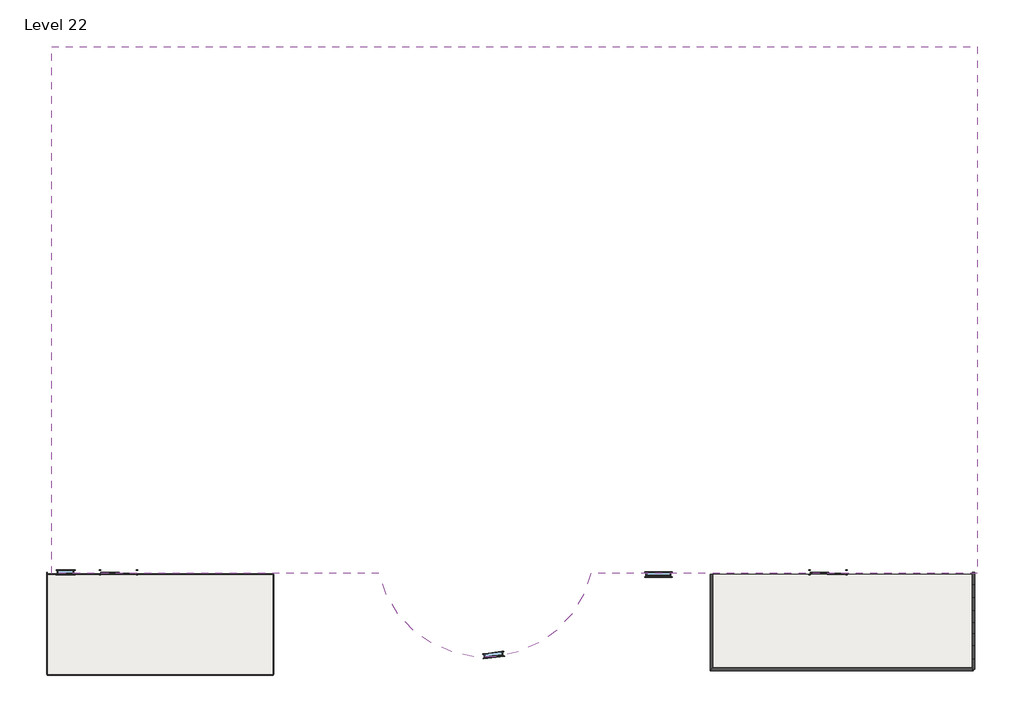
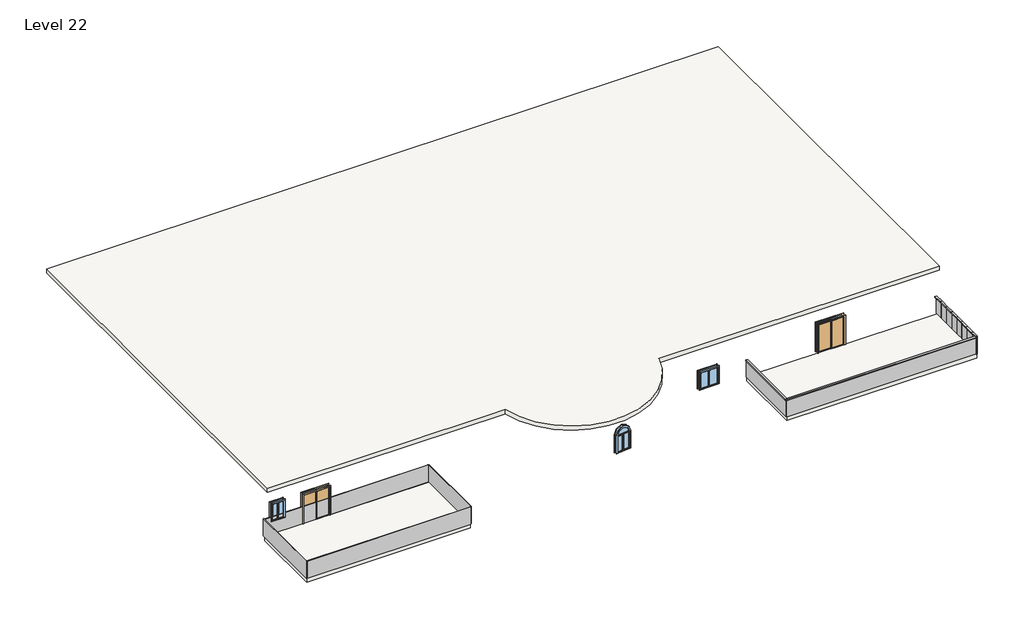
# One storey: 14 plates, 11 members, 3 slabs, 3 windows, 2 doors.
"""IFC4 building model written with IfcOpenShell, lengths in millimetres."""

from ifc_helpers import new_model, si_unit, point, frame, frame_2d, origin, place, context, project, spatial, polyline, circle_curve, trimmed, segment, composite_curve, outline, extrude, transform, mapped, element, save
from components import door_076b30e0, member_75074519, member_47bfaf8a, member_d3852687, member_b73aa13b, member_b281fab0, member_86d06fe4, member_19d8ec5e, member_fc2d78a3, system_panel_glazed_febc6b86, system_panel_glazed_7af1c9c3, system_panel_glazed_73c284ea, system_panel_glazed_3baf32ff, system_panel_glazed_cd2dd794, system_panel_glazed_8f98839e, system_panel_glazed_0c1985eb, system_panel_glazed_b96adab1, system_panel_glazed_fa2f7082, system_panel_glazed_a1141da7, window_cf4adaea, window_bb17773d, window_0862ab64

model = new_model("IFC4")

# Units and contexts
model_context = context("Model", 3, world=origin())
ifc_project = project(units=[si_unit("LENGTHUNIT", "METRE", prefix="MILLI")], contexts=[model_context])

# Site, building, storey
site = spatial("IfcSite", under=ifc_project)
building = spatial("IfcBuilding", under=site)
storey = spatial("IfcBuildingStorey", under=building, Name="Level 22", Elevation=36576.0)

# Doors
placement = place(None, origin())
door_shape = door_076b30e0(model_context)
element("IfcDoor", 1, ObjectType="Door-Double-Sliding : 68\" x 80\"", at=placement, inside=storey, context=model_context, shape_type="MappedRepresentation", body=[
    mapped(door_shape, transform((-16343.985279, -12227.7237084, 36576.0), x_axis=(-1.0, 0.0, 0.0), y_axis=(0.0, -1.0, 0.0), z_axis=(0.0, 0.0, 1.0))),
])
element("IfcDoor", 2, ObjectType="Door-Double-Sliding : 68\" x 80\"", at=placement, inside=storey, context=model_context, shape_type="MappedRepresentation", body=[
    mapped(door_shape, transform((18377.814721, -12227.7237084, 36576.0), x_axis=(-1.0, 0.0, 0.0), y_axis=(0.0, -1.0, 0.0), z_axis=(0.0, 0.0, 1.0))),
])

# Members
member_shape = member_75074519(model_context)
element("IfcMember", 3, ObjectType="Rectangular Mullion : 2.5\" x 5\" rectangular", at=placement, inside=storey, context=model_context, shape_type="MappedRepresentation", body=[
    mapped(member_shape, transform((25489.814721, -17095.151951, 37795.2), x_axis=(1.0, 0.0, 0.0), y_axis=(0.0, 1.0, 0.0), z_axis=(0.0, 0.0, 1.0))),
])
member_2_shape = member_47bfaf8a(model_context)
element("IfcMember", 4, ObjectType="Rectangular Mullion : 2.5\" x 5\" rectangular", at=placement, inside=storey, context=model_context, shape_type="MappedRepresentation", body=[
    mapped(member_2_shape, transform((25489.814721, -14809.151951, 37795.2), x_axis=(0.0, 0.0, 1.0), y_axis=(-1.0, 0.0, 0.0), z_axis=(0.0, -1.0, 0.0))),
])
element("IfcMember", 5, ObjectType="Rectangular Mullion : 2.5\" x 5\" rectangular", at=placement, inside=storey, context=model_context, shape_type="MappedRepresentation", body=[
    mapped(member_2_shape, transform((25489.814721, -15952.151951, 37795.2), x_axis=(0.0, 0.0, 1.0), y_axis=(-1.0, 0.0, 0.0), z_axis=(0.0, -1.0, 0.0))),
])
member_3_shape = member_d3852687(model_context)
element("IfcMember", 6, ObjectType="Rectangular Mullion : 2.5\" x 5\" rectangular", at=placement, inside=storey, context=model_context, shape_type="MappedRepresentation", body=[
    mapped(member_3_shape, transform((25489.814721, -16612.551951, 37795.2), x_axis=(0.0, 0.0, 1.0), y_axis=(-1.0, 0.0, 0.0), z_axis=(0.0, -1.0, 0.0))),
])
member_4_shape = member_b73aa13b(model_context)
element("IfcMember", 7, ObjectType="Rectangular Mullion : 2.5\" x 5\" rectangular", at=placement, inside=storey, context=model_context, shape_type="MappedRepresentation", body=[
    mapped(member_4_shape, transform((25489.814721, -12969.6664559, 37795.2), x_axis=(0.0, 0.0, 1.0), y_axis=(-1.0, 0.0, 0.0), z_axis=(0.0, -1.0, 0.0))),
])
element("IfcMember", 8, ObjectType="Rectangular Mullion : 2.5\" x 5\" rectangular", at=placement, inside=storey, context=model_context, shape_type="MappedRepresentation", body=[
    mapped(member_4_shape, transform((25489.814721, -13584.6092034, 37795.2), x_axis=(0.0, 0.0, 1.0), y_axis=(-1.0, 0.0, 0.0), z_axis=(0.0, -1.0, 0.0))),
])
element("IfcMember", 9, ObjectType="Rectangular Mullion : 2.5\" x 5\" rectangular", at=placement, inside=storey, context=model_context, shape_type="MappedRepresentation", body=[
    mapped(member_4_shape, transform((25489.814721, -14199.551951, 37795.2), x_axis=(0.0, 0.0, 1.0), y_axis=(-1.0, 0.0, 0.0), z_axis=(0.0, -1.0, 0.0))),
])
member_5_shape = member_b281fab0(model_context)
element("IfcMember", 10, ObjectType="Rectangular Mullion : 2.5\" x 5\" rectangular", at=placement, inside=storey, context=model_context, shape_type="MappedRepresentation", body=[
    mapped(member_5_shape, transform((25489.814721, -15342.551951, 37795.2), x_axis=(0.0, 0.0, 1.0), y_axis=(-1.0, 0.0, 0.0), z_axis=(0.0, -1.0, 0.0))),
])
member_6_shape = member_86d06fe4(model_context)
element("IfcMember", 11, ObjectType="Rectangular Mullion : 2.5\" x 5\" rectangular", at=placement, inside=storey, context=model_context, shape_type="MappedRepresentation", body=[
    mapped(member_6_shape, transform((25489.814721, -17095.151951, 37795.2), x_axis=(0.0, 0.0, 1.0), y_axis=(-1.0, 0.0, 0.0), z_axis=(0.0, -1.0, 0.0))),
])
member_7_shape = member_19d8ec5e(model_context)
element("IfcMember", 12, ObjectType="Rectangular Mullion : 2.5\" x 5\" rectangular", at=placement, inside=storey, context=model_context, shape_type="MappedRepresentation", body=[
    mapped(member_7_shape, transform((12667.5594464, -17095.151951, 37795.2), x_axis=(0.0, 0.0, 1.0), y_axis=(0.0, 1.0, 0.0), z_axis=(-1.0, 0.0, 0.0))),
])
member_8_shape = member_fc2d78a3(model_context)
element("IfcMember", 13, ObjectType="Rectangular Mullion : 2.5\" x 5\" rectangular", at=placement, inside=storey, context=model_context, shape_type="MappedRepresentation", body=[
    mapped(member_8_shape, transform((12667.5594464, -12456.3237084, 37795.2), x_axis=(0.0, 0.0, 1.0), y_axis=(1.0, 0.0, 0.0), z_axis=(0.0, 1.0, 0.0))),
])

# Plates
system_panel_glazed_shape = system_panel_glazed_febc6b86(model_context)
element("IfcPlate", 14, ObjectType="System Panel : Glazed", at=placement, inside=storey, context=model_context, shape_type="MappedRepresentation", body=[
    mapped(system_panel_glazed_shape, transform((19046.9370837, -17095.151951, 36576.0), x_axis=(-1.0, 0.0, 0.0), y_axis=(0.0, -1.0, 0.0), z_axis=(0.0, 0.0, 1.0))),
])
system_panel_glazed_2_shape = system_panel_glazed_7af1c9c3(model_context)
element("IfcPlate", 15, ObjectType="System Panel : Glazed", at=placement, inside=storey, context=model_context, shape_type="MappedRepresentation", body=[
    mapped(system_panel_glazed_2_shape, transform((25489.814721, -15647.351951, 36576.0), x_axis=(0.0, -1.0, 0.0), y_axis=(1.0, 0.0, 0.0), z_axis=(0.0, 0.0, 1.0))),
])
element("IfcPlate", 16, ObjectType="System Panel : Glazed", at=placement, inside=storey, context=model_context, shape_type="MappedRepresentation", body=[
    mapped(system_panel_glazed_2_shape, transform((25489.814721, -14504.351951, 36576.0), x_axis=(0.0, -1.0, 0.0), y_axis=(1.0, 0.0, 0.0), z_axis=(0.0, 0.0, 1.0))),
])
system_panel_glazed_3_shape = system_panel_glazed_73c284ea(model_context)
element("IfcPlate", 17, ObjectType="System Panel : Glazed", at=placement, inside=storey, context=model_context, shape_type="MappedRepresentation", body=[
    mapped(system_panel_glazed_3_shape, transform((25489.814721, -16282.351951, 36576.0), x_axis=(0.0, -1.0, 0.0), y_axis=(1.0, 0.0, 0.0), z_axis=(0.0, 0.0, 1.0))),
])
system_panel_glazed_4_shape = system_panel_glazed_3baf32ff(model_context)
element("IfcPlate", 18, ObjectType="System Panel : Glazed", at=placement, inside=storey, context=model_context, shape_type="MappedRepresentation", body=[
    mapped(system_panel_glazed_4_shape, transform((25489.814721, -12662.1950821, 36576.0), x_axis=(0.0, -1.0, 0.0), y_axis=(1.0, 0.0, 0.0), z_axis=(0.0, 0.0, 1.0))),
])
element("IfcPlate", 19, ObjectType="System Panel : Glazed", at=placement, inside=storey, context=model_context, shape_type="MappedRepresentation", body=[
    mapped(system_panel_glazed_4_shape, transform((25489.814721, -13892.0805772, 36576.0), x_axis=(0.0, -1.0, 0.0), y_axis=(1.0, 0.0, 0.0), z_axis=(0.0, 0.0, 1.0))),
])
element("IfcPlate", 20, ObjectType="System Panel : Glazed", at=placement, inside=storey, context=model_context, shape_type="MappedRepresentation", body=[
    mapped(system_panel_glazed_4_shape, transform((25489.814721, -13277.1378297, 36576.0), x_axis=(0.0, -1.0, 0.0), y_axis=(1.0, 0.0, 0.0), z_axis=(0.0, 0.0, 1.0))),
])
system_panel_glazed_5_shape = system_panel_glazed_cd2dd794(model_context)
element("IfcPlate", 21, ObjectType="System Panel : Glazed", at=placement, inside=storey, context=model_context, shape_type="MappedRepresentation", body=[
    mapped(system_panel_glazed_5_shape, transform((25489.814721, -16853.851951, 36576.0), x_axis=(0.0, -1.0, 0.0), y_axis=(1.0, 0.0, 0.0), z_axis=(0.0, 0.0, 1.0))),
])
system_panel_glazed_6_shape = system_panel_glazed_8f98839e(model_context)
element("IfcPlate", 22, ObjectType="System Panel : Glazed", at=placement, inside=storey, context=model_context, shape_type="MappedRepresentation", body=[
    mapped(system_panel_glazed_6_shape, transform((25489.814721, -15075.851951, 36576.0), x_axis=(0.0, -1.0, 0.0), y_axis=(1.0, 0.0, 0.0), z_axis=(0.0, 0.0, 1.0))),
])
system_panel_glazed_7_shape = system_panel_glazed_0c1985eb(model_context)
element("IfcPlate", 23, ObjectType="System Panel : Glazed", at=placement, inside=storey, context=model_context, shape_type="MappedRepresentation", body=[
    mapped(system_panel_glazed_7_shape, transform((12667.5594464, -14775.7378297, 36576.0), x_axis=(0.0, 1.0, 0.0), y_axis=(-1.0, 0.0, 0.0), z_axis=(0.0, 0.0, 1.0))),
])
system_panel_glazed_8_shape = system_panel_glazed_b96adab1(model_context)
element("IfcPlate", 24, ObjectType="System Panel : Glazed", at=placement, inside=storey, context=model_context, shape_type="MappedRepresentation", body=[
    mapped(system_panel_glazed_8_shape, transform((-14302.7926538, -12456.3237084, 36576.0), x_axis=(1.0, 0.0, 0.0), y_axis=(0.0, 1.0, 0.0), z_axis=(0.0, 0.0, 1.0))),
])
element("IfcPlate", 25, ObjectType="System Panel : Glazed", at=placement, inside=storey, context=model_context, shape_type="MappedRepresentation", body=[
    mapped(system_panel_glazed_8_shape, transform((-14302.7926538, -17340.4434729, 36576.0), x_axis=(-1.0, 0.0, 0.0), y_axis=(0.0, -1.0, 0.0), z_axis=(0.0, 0.0, 1.0))),
])
system_panel_glazed_9_shape = system_panel_glazed_fa2f7082(model_context)
element("IfcPlate", 26, ObjectType="System Panel : Glazed", at=placement, inside=storey, context=model_context, shape_type="MappedRepresentation", body=[
    mapped(system_panel_glazed_9_shape, transform((-8781.8000285, -14898.3835906, 36576.0), x_axis=(0.0, -1.0, 0.0), y_axis=(1.0, 0.0, 0.0), z_axis=(0.0, 0.0, 1.0))),
])
system_panel_glazed_10_shape = system_panel_glazed_a1141da7(model_context)
element("IfcPlate", 27, ObjectType="System Panel : Glazed", at=placement, inside=storey, context=model_context, shape_type="MappedRepresentation", body=[
    mapped(system_panel_glazed_10_shape, transform((-19823.785279, -14847.5835906, 36576.0), x_axis=(0.0, 1.0, 0.0), y_axis=(-1.0, 0.0, 0.0), z_axis=(0.0, 0.0, 1.0))),
])

# Slabs
element("IfcSlab", 28, ObjectType="Generic - 12\"", at=placement, inside=storey, context=model_context, shape_type="SweptSolid", body=[
    extrude(outline(composite_curve([segment(polyline([(25693.014721, 13405.0447861), (25693.014721, -12401.3552139), (6774.7594464, -12401.3552139)]), True, "CONTINUOUS"), segment(trimmed(circle_curve(frame_2d((1588.414721, -11170.7221727)), 5330.3498284), [point((6774.7594464, -12401.3552139))], [point((-3597.9300045, -12401.3552139))], False, "CARTESIAN"), True, "CONTINUOUS"), segment(polyline([(-3597.9300045, -12401.3552139), (-19620.585279, -12401.3552139), (-19620.585279, 13405.0447861), (25693.014721, 13405.0447861)]), True, "CONTINUOUS")], self_intersect=False)), frame((0.0, 0.0, 39610.8098476), z_axis=(0.0, 0.0, 1.0), x_axis=(1.0, 0.0, 0.0)), (0.0, 0.0, 1.0), 304.8),
])
element("IfcSlab", 29, ObjectType="Generic - 12\"", at=placement, inside=storey, context=model_context, shape_type="SweptSolid", body=[
    extrude(outline(polyline([(25489.814721, -12434.5091907), (25489.814721, -17095.151951), (12690.685965, -17095.151951), (12690.685965, -12434.5091907), (25489.814721, -12434.5091907)])), frame((0.0, 0.0, 36271.2), z_axis=(0.0, 0.0, 1.0), x_axis=(1.0, 0.0, 0.0)), (0.0, 0.0, 1.0), 304.8),
])
element("IfcSlab", 30, ObjectType="Generic - 12\"", at=placement, inside=storey, context=model_context, shape_type="SweptSolid", body=[
    extrude(outline(polyline([(-8781.8000285, -12456.3237084), (-8781.8000285, -17340.4434729), (-19823.785279, -17340.4434729), (-19823.785279, -12456.3237084), (-8781.8000285, -12456.3237084)])), frame((0.0, 0.0, 36271.2), z_axis=(0.0, 0.0, 1.0), x_axis=(1.0, 0.0, 0.0)), (0.0, 0.0, 1.0), 304.8),
])

# Windows
window_shape = window_cf4adaea(model_context)
element("IfcWindow", 31, ObjectType="36\" x 48\"", at=placement, inside=storey, context=model_context, shape_type="MappedRepresentation", body=[
    mapped(window_shape, transform((2015.9502582, -16396.4760316, 36576.0), x_axis=(-0.9928272065785434, -0.11955809415278516, 0.0), y_axis=(0.11955809415278516, -0.9928272065785434, 0.0), z_axis=(0.0, 0.0, 1.0))),
])
window_2_shape = window_bb17773d(model_context)
element("IfcWindow", 32, ObjectType="Casement Dbl with Trim : 32\" x 48\"", at=placement, inside=storey, context=model_context, shape_type="MappedRepresentation", body=[
    mapped(window_2_shape, transform((-18934.785279, -12335.6737084, 36576.0), x_axis=(-1.0, 0.0, 0.0), y_axis=(0.0, -1.0, 0.0), z_axis=(0.0, 0.0, 1.0))),
])
window_3_shape = window_0862ab64(model_context)
element("IfcWindow", 33, ObjectType="Casement Dbl with Trim : 48\" x 48\"", at=placement, inside=storey, context=model_context, shape_type="MappedRepresentation", body=[
    mapped(window_3_shape, transform((10076.7594464, -12437.2737084, 35930.4788406), x_axis=(-1.0, 0.0, 0.0), y_axis=(0.0, -1.0, 0.0), z_axis=(0.0, 0.0, 1.0))),
])

save(model, "model.ifc")

# Revit data of these elements
# Type "Door-Double-Sliding : 68\" x 80\""
#   Type Mark = "10"
#   Construction Type Id = "opn-d45"
#   Assembly Code = "C1020"
#   Analytic Construction = "Wood frame, double glass door "
#   Thickness = 0' - 2"
#   Thermal Resistance (R) = 1.8150 (h·ft²·°F)/BTU
#   Heat Transfer Coefficient (U) = 0.5510 BTU/(h·ft²·°F)
#   Height = 6' - 8"
#   Rail Width = 0' - 2"
#   Stiles = 0' - 2"
#   Trim Projection Ext = 0' - 1"
#   Trim Projection Int = 0' - 1"
#   Trim Width = 0' - 3"
#   Width = 5' - 8"
#   Define Thermal Properties by = 1
#   Glazing = Glass
#   Panel Material = Wood - Birch - Solid Stained Light Low Gloss
#   Trim Material = Paint - Sienna
#   Visual Light Transmittance = 0
#   Solar Heat Gain Coefficient = 0
#   Function = (empty or 0)
#   Wall Closure = (empty or 0)
# Type "Rectangular Mullion : 2.5\" x 5\" rectangular"
#   built-in parameter 1007304 = 0.416667 (stored number, unit not read)
#   built-in parameter 1007301 = 0.104167 (stored number, unit not read)
#   built-in parameter 1007300 = 0.104167 (stored number, unit not read)
# Type "System Panel : Glazed"
#   Construction Type Id = "GSP4R"
#   Analytic Construction = "1/8 in Pilkington single glazing"
#   Visual Light Transmittance = 0.9
#   Solar Heat Gain Coefficient = 0.86
#   Heat Transfer Coefficient (U) = 1.18115 BTU/(h·ft²·°F)
# Type "Generic - 12\""
#   Assembly Code = "B1010"
#   Function = 0
#   Layers, outside or top first: 1' - 0" no material (function 1)
# Type "36\" x 48\""
#   Type Mark = "38"
#   Construction Type Id = "SGL"
#   Assembly Code = "B2020100"
#   Analytic Construction = "Large single-glazed windows"
#   Visual Light Transmittance = 0.9
#   Solar Heat Gain Coefficient = 0.86
#   Heat Transfer Coefficient (U) = 0.979472 BTU/(h·ft²·°F)
#   Height = 4' - 0"
#   Default Sill Height = 3' - 0"
#   Trim Projection - Ext. = 0' - 0 1/2"
#   Trim Projection - Int. = 0' - 0 3/4"
#   Trim Width - Exterior = 0' - 3 1/2"
#   Trim Width - Interior = 0' - 3 1/2"
#   Width = 3' - 0"
#   Window Inset = 0' - 0 3/4"
#   Define Thermal Properties by = 1
#   Glass Pane Material = Glass
#   Sash Material = Sash
#   Trim Exterior Material = Trim
#   Trim Interior Material = Trim
#   Wall Closure = (empty or 0)
# Type "Casement Dbl with Trim : 32\" x 48\""
#   Type Mark = "36"
#   Construction Type Id = "GSP4R"
#   Assembly Code = "B2020100"
#   Analytic Construction = "1/8 in Pilkington single glazing"
#   Visual Light Transmittance = 0.9
#   Solar Heat Gain Coefficient = 0.78
#   Heat Transfer Coefficient (U) = 0.6496 BTU/(h·ft²·°F)
#   Height = 4' - 0"
#   Default Sill Height = 3' - 0"
#   Trim Projection - Ext. = 0' - 0 1/2"
#   Trim Projection - Int. = 0' - 0 3/4"
#   Trim Width - Exterior = 0' - 3 1/2"
#   Trim Width - Interior = 0' - 3 1/2"
#   Width = 2' - 8"
#   Window Inset = 0' - 0 3/4"
#   Define Thermal Properties by = 1
#   Glass Pane Material = Glass
#   Sash Material = Sash
#   Trim Exterior Material = Trim
#   Trim Interior Material = Trim
#   Wall Closure = (empty or 0)
# Type "Casement Dbl with Trim : 48\" x 48\""
#   Type Mark = "34"
#   Construction Type Id = "GSP4R"
#   Assembly Code = "B2020100"
#   Analytic Construction = "1/8 in Pilkington single glazing"
#   Visual Light Transmittance = 0.9
#   Solar Heat Gain Coefficient = 0.78
#   Heat Transfer Coefficient (U) = 0.6496 BTU/(h·ft²·°F)
#   Height = 4' - 0"
#   Default Sill Height = 3' - 0"
#   Trim Projection - Ext. = 0' - 0 1/2"
#   Trim Projection - Int. = 0' - 0 3/4"
#   Trim Width - Exterior = 0' - 3 1/2"
#   Trim Width - Interior = 0' - 3 1/2"
#   Width = 4' - 0"
#   Window Inset = 0' - 0 3/4"
#   Define Thermal Properties by = 1
#   Glass Pane Material = Glass
#   Sash Material = Sash
#   Trim Exterior Material = Trim
#   Trim Interior Material = Trim
#   Wall Closure = (empty or 0)
# Elements 1, 2 (IfcDoor, "Door-Double-Sliding : 68\" x 80\"")
#   Phase Created = New Construction
#   Materials on its faces: "Paint - Sienna", "Wood - Birch - Solid Stained Light Low Gloss", "Glass"
# Elements 3, 4, 5, 6, 7, 8, 9, 10, 11, 12, 13 (IfcMember, "Rectangular Mullion : 2.5\" x 5\" rectangular")
#   Phase Created = New Construction
#   Materials on its faces: "Aluminum"
# Elements 14, 15, 16, 17, 18, 19, 20, 21, 22, 23, 24, 25, 26, 27 (IfcPlate, "System Panel : Glazed")
#   Phase Created = New Construction
#   Materials on its faces: "Glass"
# Element 28 (IfcSlab, "Generic - 12\"")
#   Height Offset From Level = 10' - 11.4807"
#   Phase Created = New Construction
#   Materials on its faces: "Default Floor"
# Elements 29, 30 (IfcSlab, "Generic - 12\"")
#   Height Offset From Level = 0' - 0"
#   Phase Created = New Construction
#   Materials on its faces: "Default Floor"
# Element 31 (IfcWindow, "36\" x 48\"")
#   Mark = "23"
#   Phase Created = New Construction
#   Materials on its faces: "Sash", "Trim", "Glass"
# Element 32 (IfcWindow, "Casement Dbl with Trim : 32\" x 48\"")
#   Mark = "40"
#   Phase Created = New Construction
#   Materials on its faces: "Sash", "Trim", "Glass"
# Element 33 (IfcWindow, "Casement Dbl with Trim : 48\" x 48\"")
#   Mark = "6"
#   Phase Created = New Construction
#   Materials on its faces: "Sash", "Trim", "Glass"
# Materials
#   "Glass": class "Glass", colour RGB 0 128 192, transparency 0.75, Description = "Soda Lime Glass", Cost = 0
#   "Wood - Birch - Solid Stained Light Low Gloss": class "Wood", colour RGB 210 159 95, transparency 0, Cost = 0
#   "Paint - Sienna": colour RGB 118 70 51, transparency 0, Cost = 0
#   "Sash": class "Wood", colour RGB 224 178 126, transparency 0
#   "Trim": class "Wood", colour RGB 224 178 126, transparency 0
#   "Aluminum": class "Metal", colour RGB 247 247 247, transparency 0, Description = "Aluminum 6061", Cost = 0
#   "Default Floor": colour RGB 128 128 128, transparency 0
